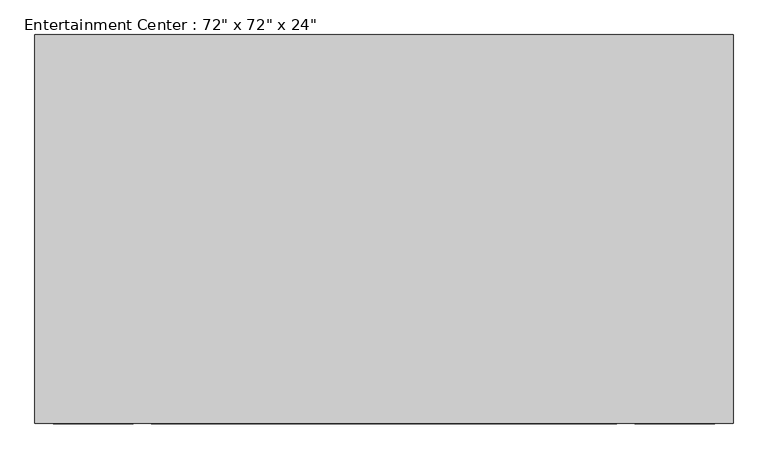
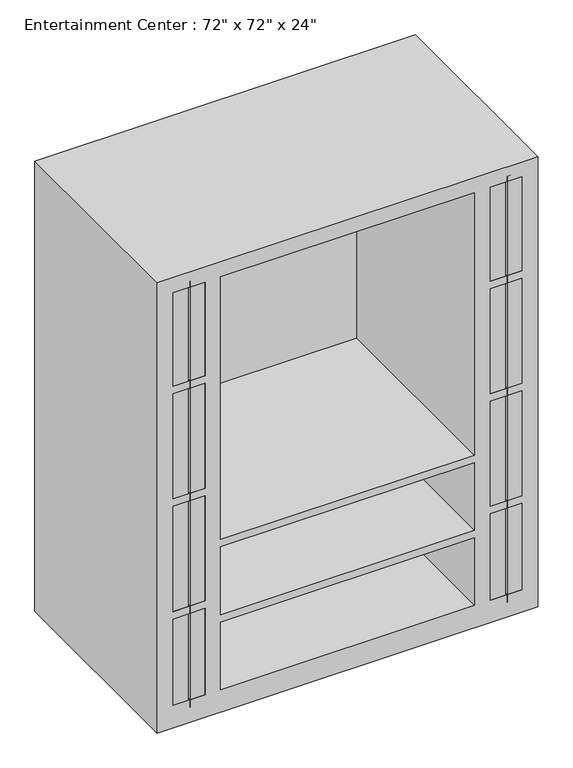
"""IFC4 building model written with IfcOpenShell, lengths in millimetres: furniture geometry."""

from ifc_helpers import new_model, si_unit, point, frame, frame_2d, origin, place, context, project, spatial, polyline, circle_curve, trimmed, segment, composite_curve, outline, extrude, faceted_brep, source, transform, mapped, element, save


def furniture_c333be35(model_context):
    return source(origin(), model_context, "Body", "SolidModel", [
        faceted_brep([(609.6, -781.05, 0.0), (609.6, -781.05, 1524.0), (-609.6, -781.05, 1524.0), (-609.6, -781.05, 0.0), (-457.2, -781.05, 1473.2), (-457.2, -781.05, 1155.7), (-558.8, -781.05, 1155.7), (-558.8, -781.05, 1473.2), (-457.2, -781.05, 76.2), (-558.8, -781.05, 76.2), (-558.8, -781.05, 368.3), (-457.2, -781.05, 368.3), (558.8, -781.05, 1155.7), (457.2, -781.05, 1155.7), (457.2, -781.05, 1473.2), (558.8, -781.05, 1473.2), (-406.4, -781.05, 584.2), (-406.4, -781.05, 1473.2), (406.4, -781.05, 1473.2), (406.4, -781.05, 584.2), (406.4, -781.05, 76.2), (-406.4, -781.05, 76.2), (-406.4, -781.05, 304.8), (406.4, -781.05, 304.8), (558.8, -781.05, 76.2), (457.2, -781.05, 76.2), (457.2, -781.05, 368.3), (558.8, -781.05, 368.3), (-558.8, -781.05, 393.7), (-558.8, -781.05, 749.3), (-457.2, -781.05, 749.3), (-457.2, -781.05, 393.7), (-457.2, -781.05, 1130.3), (-457.2, -781.05, 774.7), (-558.8, -781.05, 774.7), (-558.8, -781.05, 1130.3), (457.2, -781.05, 1130.3), (558.8, -781.05, 1130.3), (558.8, -781.05, 774.7), (457.2, -781.05, 774.7), (457.2, -781.05, 749.3), (558.8, -781.05, 749.3), (558.8, -781.05, 393.7), (457.2, -781.05, 393.7), (406.4, -781.05, 330.2), (-406.4, -781.05, 330.2), (-406.4, -781.05, 558.8), (406.4, -781.05, 558.8), (609.6, -101.6, 0.0), (-609.6, -101.6, 0.0), (-609.6, -101.6, 1524.0), (609.6, -101.6, 1524.0), (-457.2, -127.0, 1473.2), (-457.2, -127.0, 1155.7), (-558.8, -127.0, 1155.7), (-558.8, -127.0, 1473.2), (-457.2, -127.0, 76.2), (-558.8, -127.0, 76.2), (-558.8, -127.0, 368.3), (-457.2, -127.0, 368.3), (558.8, -127.0, 1155.7), (457.2, -127.0, 1155.7), (457.2, -127.0, 1473.2), (558.8, -127.0, 1473.2), (-406.4, -127.0, 584.2), (-406.4, -127.0, 1473.2), (406.4, -127.0, 1473.2), (406.4, -127.0, 584.2), (406.4, -127.0, 76.2), (-406.4, -127.0, 76.2), (-406.4, -127.0, 304.8), (406.4, -127.0, 304.8), (558.8, -127.0, 76.2), (457.2, -127.0, 76.2), (457.2, -127.0, 368.3), (558.8, -127.0, 368.3), (-558.8, -127.0, 393.7), (-558.8, -127.0, 749.3), (-457.2, -127.0, 749.3), (-457.2, -127.0, 393.7), (-457.2, -127.0, 1130.3), (-457.2, -127.0, 774.7), (-558.8, -127.0, 774.7), (-558.8, -127.0, 1130.3), (457.2, -127.0, 1130.3), (558.8, -127.0, 1130.3), (558.8, -127.0, 774.7), (457.2, -127.0, 774.7), (457.2, -127.0, 749.3), (558.8, -127.0, 749.3), (558.8, -127.0, 393.7), (457.2, -127.0, 393.7), (406.4, -127.0, 330.2), (-406.4, -127.0, 330.2), (-406.4, -127.0, 558.8), (406.4, -127.0, 558.8)], [[[0, 1, 2, 3], [4, 5, 6, 7], [8, 9, 10, 11], [12, 13, 14, 15], [16, 17, 18, 19], [20, 21, 22, 23], [24, 25, 26, 27], [28, 29, 30, 31], [32, 33, 34, 35], [36, 37, 38, 39], [40, 41, 42, 43], [44, 45, 46, 47]], [[48, 49, 50, 51]], [[1, 0, 48, 51]], [[2, 1, 51, 50]], [[3, 2, 50, 49]], [[0, 3, 49, 48]], [[5, 4, 52, 53]], [[6, 5, 53, 54]], [[7, 6, 54, 55]], [[4, 7, 55, 52]], [[9, 8, 56, 57]], [[10, 9, 57, 58]], [[11, 10, 58, 59]], [[8, 11, 59, 56]], [[13, 12, 60, 61]], [[14, 13, 61, 62]], [[15, 14, 62, 63]], [[12, 15, 63, 60]], [[17, 16, 64, 65]], [[18, 17, 65, 66]], [[19, 18, 66, 67]], [[16, 19, 67, 64]], [[21, 20, 68, 69]], [[22, 21, 69, 70]], [[23, 22, 70, 71]], [[20, 23, 71, 68]], [[25, 24, 72, 73]], [[26, 25, 73, 74]], [[27, 26, 74, 75]], [[24, 27, 75, 72]], [[29, 28, 76, 77]], [[30, 29, 77, 78]], [[31, 30, 78, 79]], [[28, 31, 79, 76]], [[33, 32, 80, 81]], [[34, 33, 81, 82]], [[35, 34, 82, 83]], [[32, 35, 83, 80]], [[37, 36, 84, 85]], [[38, 37, 85, 86]], [[39, 38, 86, 87]], [[36, 39, 87, 84]], [[41, 40, 88, 89]], [[42, 41, 89, 90]], [[43, 42, 90, 91]], [[40, 43, 91, 88]], [[45, 44, 92, 93]], [[46, 45, 93, 94]], [[47, 46, 94, 95]], [[44, 47, 95, 92]], [[53, 52, 55, 54]], [[57, 56, 59, 58]], [[61, 60, 63, 62]], [[65, 64, 67, 66]], [[69, 68, 71, 70]], [[73, 72, 75, 74]], [[77, 76, 79, 78]], [[81, 80, 83, 82]], [[85, 84, 87, 86]], [[89, 88, 91, 90]], [[93, 92, 95, 94]]]),
        extrude(outline(composite_curve([segment(polyline([(850.9, -480.5986452), (850.9, -504.825), (673.1, -504.825), (673.1, -480.5986452)]), True, "CONTINUOUS"), segment(trimmed(circle_curve(frame_2d((698.5, -480.5986452)), 25.4), [point((673.1, -480.5986452))], [point((698.5, -455.1986452))], False, "CARTESIAN"), True, "CONTINUOUS"), segment(polyline([(698.5, -455.1986452), (825.5, -455.1986452)]), True, "CONTINUOUS"), segment(trimmed(circle_curve(frame_2d((825.5, -480.5986452)), 25.4), [point((825.5, -455.1986452))], [point((850.9, -480.5986452))], False, "CARTESIAN"), True, "CONTINUOUS")], self_intersect=False)), frame((0.0, -714.375, 0.0), z_axis=(0.0, 1.0, 0.0), x_axis=(0.0, 0.0, 1.0)), (0.0, 0.0, 1.0), 3.175),
        extrude(outline(composite_curve([segment(trimmed(circle_curve(frame_2d((825.5, -535.78125)), 25.4), [point((850.9, -535.78125))], [point((825.5, -561.18125))], False, "CARTESIAN"), True, "CONTINUOUS"), segment(polyline([(825.5, -561.18125), (698.5, -561.18125)]), True, "CONTINUOUS"), segment(trimmed(circle_curve(frame_2d((698.5, -535.78125)), 25.4), [point((698.5, -561.18125))], [point((673.1, -535.78125))], False, "CARTESIAN"), True, "CONTINUOUS"), segment(polyline([(673.1, -535.78125), (673.1, -511.175), (850.9, -511.175), (850.9, -535.78125)]), True, "CONTINUOUS")], self_intersect=False)), frame((0.0, -714.375, 0.0), z_axis=(0.0, 1.0, 0.0), x_axis=(0.0, 0.0, 1.0)), (0.0, 0.0, 1.0), 3.175),
        extrude(outline(composite_curve([segment(trimmed(circle_curve(frame_2d((825.5, 480.5986452)), 25.4), [point((850.9, 480.5986452))], [point((825.5, 455.1986452))], False, "CARTESIAN"), True, "CONTINUOUS"), segment(polyline([(825.5, 455.1986452), (698.5, 455.1986452)]), True, "CONTINUOUS"), segment(trimmed(circle_curve(frame_2d((698.5, 480.5986452)), 25.4), [point((698.5, 455.1986452))], [point((673.1, 480.5986452))], False, "CARTESIAN"), True, "CONTINUOUS"), segment(polyline([(673.1, 480.5986452), (673.1, 504.825), (850.9, 504.825), (850.9, 480.5986452)]), True, "CONTINUOUS")], self_intersect=False)), frame((0.0, -714.375, 0.0), z_axis=(0.0, 1.0, 0.0), x_axis=(0.0, 0.0, 1.0)), (0.0, 0.0, 1.0), 3.175),
        extrude(outline(composite_curve([segment(polyline([(850.9, 535.78125), (850.9, 511.175), (673.1, 511.175), (673.1, 535.78125)]), True, "CONTINUOUS"), segment(trimmed(circle_curve(frame_2d((698.5, 535.78125)), 25.4), [point((673.1, 535.78125))], [point((698.5, 561.18125))], False, "CARTESIAN"), True, "CONTINUOUS"), segment(polyline([(698.5, 561.18125), (825.5, 561.18125)]), True, "CONTINUOUS"), segment(trimmed(circle_curve(frame_2d((825.5, 535.78125)), 25.4), [point((825.5, 561.18125))], [point((850.9, 535.78125))], False, "CARTESIAN"), True, "CONTINUOUS")], self_intersect=False)), frame((0.0, -714.375, 0.0), z_axis=(0.0, 1.0, 0.0), x_axis=(0.0, 0.0, 1.0)), (0.0, 0.0, 1.0), 3.175),
        extrude(outline(polyline([(-577.85, -711.2), (-511.175, -711.2), (-511.175, -781.05), (-577.85, -781.05), (-577.85, -711.2)])), frame((0.0, 0.0, 50.8), z_axis=(0.0, 0.0, 1.0), x_axis=(1.0, 0.0, 0.0)), (0.0, 0.0, 1.0), 1441.45),
        extrude(outline(polyline([(-504.825, -711.2), (-438.15, -711.2), (-438.15, -781.05), (-504.825, -781.05), (-504.825, -711.2)])), frame((0.0, 0.0, 50.8), z_axis=(0.0, 0.0, 1.0), x_axis=(1.0, 0.0, 0.0)), (0.0, 0.0, 1.0), 1441.45),
        extrude(outline(polyline([(511.175, -711.2), (577.85, -711.2), (577.85, -781.05), (511.175, -781.05), (511.175, -711.2)])), frame((0.0, 0.0, 50.8), z_axis=(0.0, 0.0, 1.0), x_axis=(1.0, 0.0, 0.0)), (0.0, 0.0, 1.0), 1441.45),
        extrude(outline(polyline([(438.15, -711.2), (504.825, -711.2), (504.825, -781.05), (438.15, -781.05), (438.15, -711.2)])), frame((0.0, 0.0, 50.8), z_axis=(0.0, 0.0, 1.0), x_axis=(1.0, 0.0, 0.0)), (0.0, 0.0, 1.0), 1441.45),
    ])


if __name__ == "__main__":
    model = new_model("IFC4")
    model_context = context("Model", 3, world=origin())
    ifc_project = project(units=[si_unit("LENGTHUNIT", "METRE", prefix="MILLI")], contexts=[model_context])
    site = spatial("IfcSite", under=ifc_project)
    building = spatial("IfcBuilding", under=site)
    placement = place(None, origin())
    furniture_shape = furniture_c333be35(model_context)
    element("IfcFurniture", 1, ObjectType="Entertainment Center : 72\" x 72\" x 24\"", at=placement, inside=building, context=model_context, shape_type="MappedRepresentation", body=[
        mapped(furniture_shape, transform((0.0, 0.0, 0.0), x_axis=(1.0, 0.0, 0.0), y_axis=(0.0, 1.0, 0.0), z_axis=(0.0, 0.0, 1.0))),
    ])
    save(model, "model.ifc")

# Revit data of these elements
# Type "Entertainment Center : 72\" x 72\" x 24\""
#   Assembly Code = "E2020200"
#   Center Width = 2' - 8"
#   Depth = 2' - 0"
#   Height = 5' - 0"
#   Width = 4' - 0"
#   Material = none
#   Default Elevation = 0
# Element 1 (IfcFurniture, "Entertainment Center : 72\" x 72\" x 24\"")
#   Materials on its faces: "Steel, Chrome Plated", "Glass - Clear, Grey"
# Materials
#   "Steel, Chrome Plated": class "Metal", colour RGB 17 17 17, transparency 0, Description = "Chromiuim plated steel", Cost = 0
#   "Glass - Clear, Grey": class "Glass", colour RGB 252 255 255, transparency 0.64
